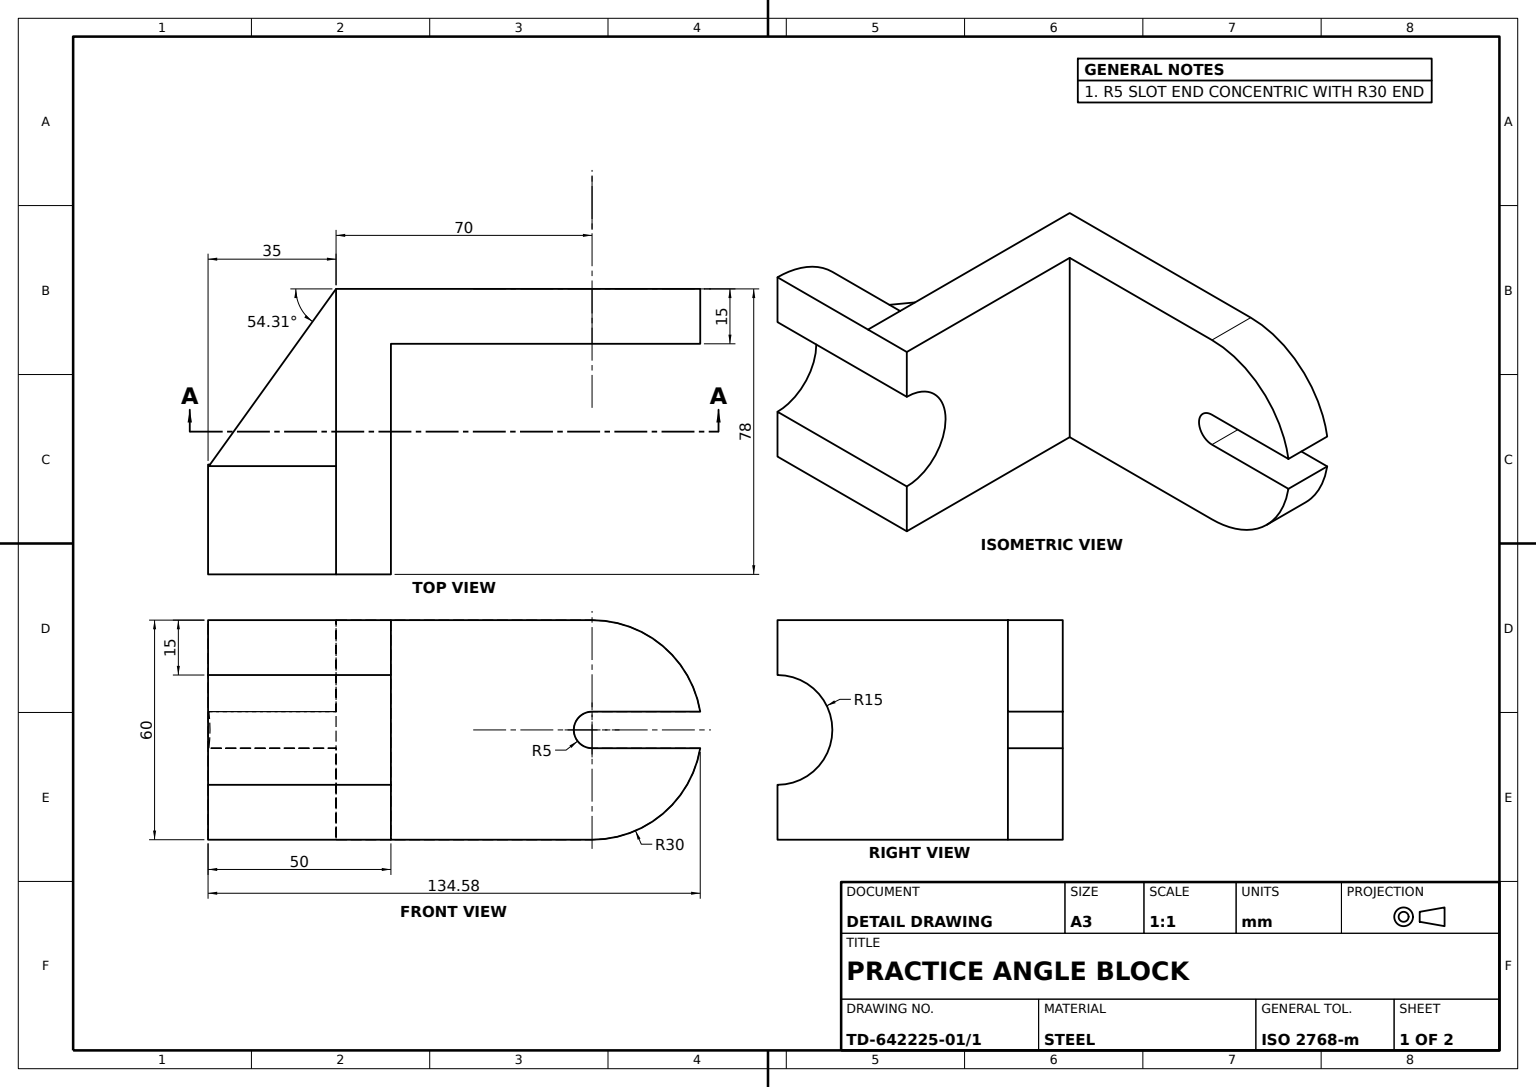
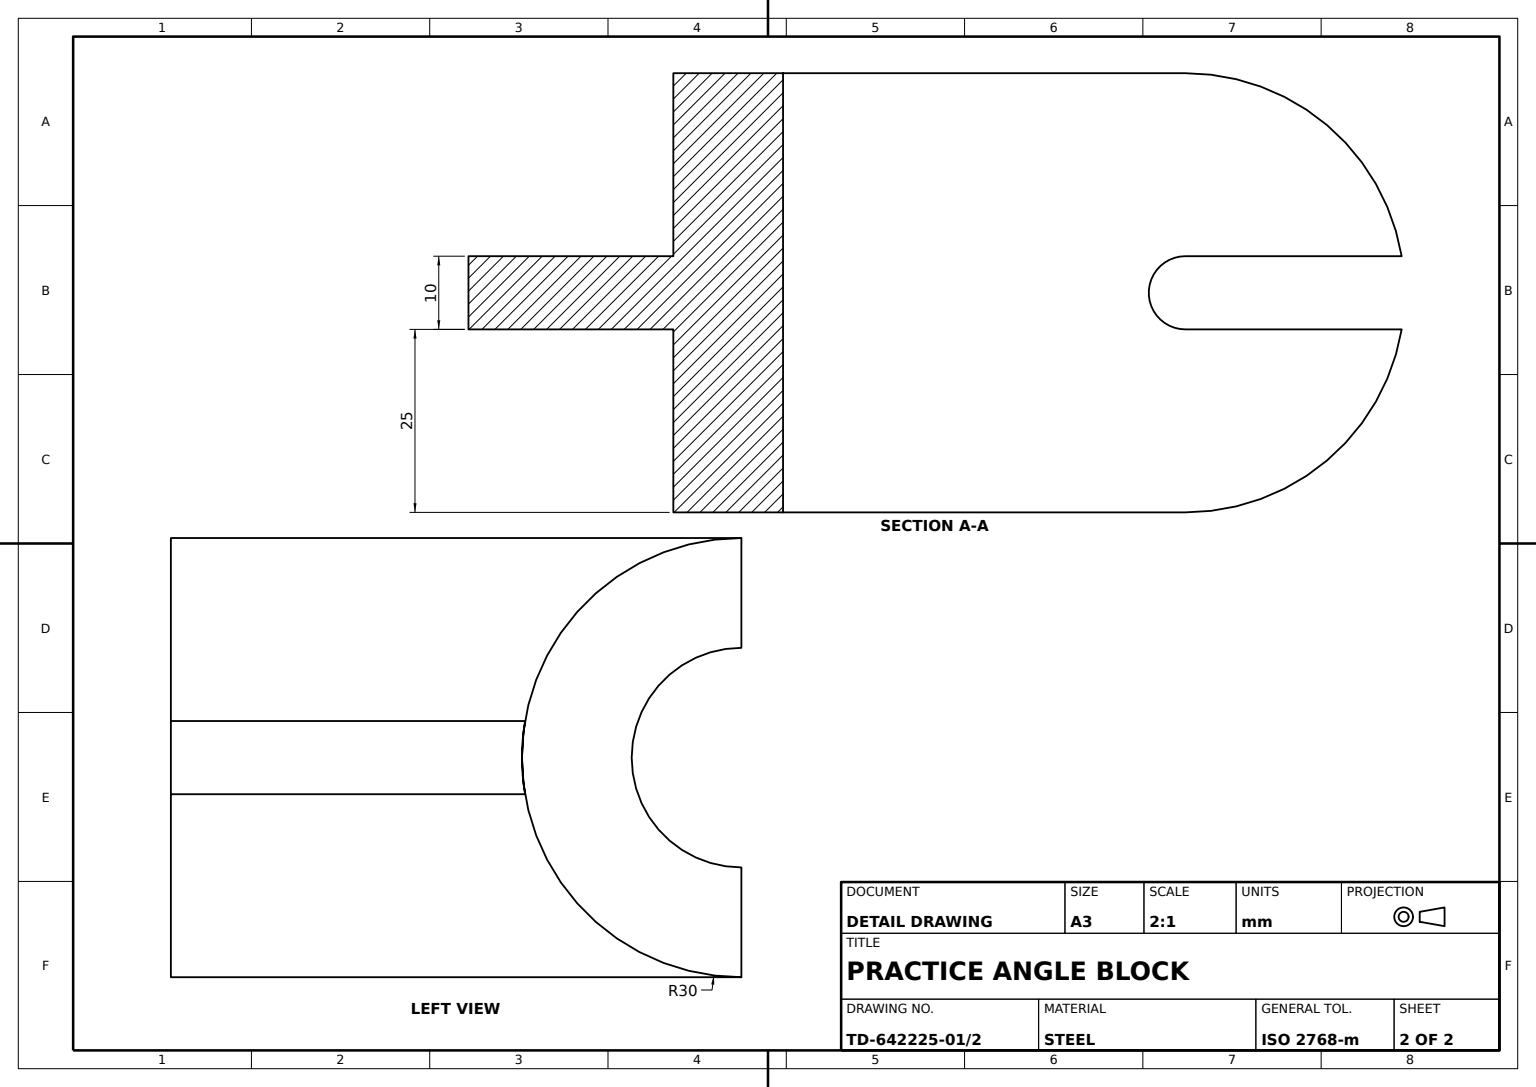
SolidWorks part; units mm, degrees
material "Plain Carbon Steel"
ref_plane "Front Plane" through (0, 0, 0) normal (0, 0, 1) x (1, 0, 0)
ref_plane "Top Plane" through (0, 0, 0) normal (0, 1, 0) x (1, 0, 0)
ref_plane "Right Plane" through (0, 0, 0) normal (1, 0, 0) x (0, 0, -1)
sketch "Base Block Sketch" plane through (0, 0, 0) normal (1, 0, 0) x (0, 0, -1)
  line L0 (0, 0) -> (70, 0)
  line L1 (70, 0) -> (70, -60)
  line L2 (70, -60) -> (0, -60)
  line L3 (0, -60) -> (0, 0)
  dimension "D1" = 60
  dimension "D2" = 70
extrude "Base Block 60x70x15" add sketch "Base Block Sketch" along normal blind 15
sketch "Upper Lug Sketch" plane through (0, 0, 0) normal (-1, 0, 0) x (0, 0, 1)
  line L0 (-70, -60) -> (-70, 0) construction
  line L1 (-70, 0) -> (-70, -60)
  arc A0 (-70, 0) -> (-70, -60) centre (-70, -30) ccw
extrude "Upper Round Lug" add sketch "Upper Lug Sketch" against normal blind 15
sketch "Upper Slot Sketch" plane through (15, 0, 0) normal (1, 0, 0) x (0, 0, -1)
  line L0 (70, -25) -> (99.5804, -25)
  line L1 (70, -35) -> (99.5804, -35)
  arc A0 (70, -25) -> (70, -35) centre (70, -30) ccw
  arc A1 (70, -60) -> (70, 0) centre (70, -30) ccw construction
  arc A2 (99.5804, -25) -> (99.5804, -35) centre (99.5804, -30) cw
  dimension "D1" = 10
extrude "Upper Slot 10mm" cut sketch "Upper Slot Sketch" against normal blind 15
sketch "Top Plate Sketch" plane through (0, 0, 0) normal (0, 0, 1) x (1, 0, 0)
  line L0 (0, 0) -> (78, 0)
  line L1 (78, 0) -> (78, -60)
  line L2 (78, -60) -> (0, -60)
  line L3 (0, -60) -> (0, 0)
  dimension "D1" = 78
extrude "Top Plate 78mm" add sketch "Top Plate Sketch" against normal blind 15
sketch "Radius Cut Sketch" plane through (0, 0, 0) normal (0, 0, 1) x (1, 0, 0)
  line L0 (78, -60) -> (78, 0) construction
  circle A0 centre (78, -30) radius 30
extrude "Radius Cut" cut sketch "Radius Cut Sketch" against normal blind 15
sketch "Lower Lug Sketch" plane through (0, 0, -15) normal (0, 0, -1) x (-1, 0, 0)
  line L0 (-78, -60) -> (-78, -45)
  line L1 (-78, -15) -> (-78, 0)
  arc A0 (-78, -60) -> (-78, 0) centre (-78, -30) ccw construction
  arc A1 (-78, -45) -> (-78, -15) centre (-78, -30) ccw
  arc A2 (-78, -60) -> (-78, 0) centre (-78, -30) ccw
  dimension "D1" = 15
  dimension "D2" = 15
  dimension "D3" = 15
extrude "Lower Lug 50mm" add sketch "Lower Lug Sketch" against normal blind 50
ref_plane "Rib Mid Plane" through (0, -30, 0) normal (0, -1, 0) x (-1, 0, 0)
sketch "Rib Sketch" plane through (0, -30, 0) normal (0, -1, 0) x (-1, 0, 0)
  line L0 (0, 0) -> (-48.734, -35)
  line L1 (-78, -35) -> (-48, -35) construction
  dimension "D1" = 60
rib "Support Rib 10mm" sketch "Rib Sketch" sketch "Rib Sketch" thickness 10 extrusion direction parallel to sketch draft on no parameters "D1"=10
